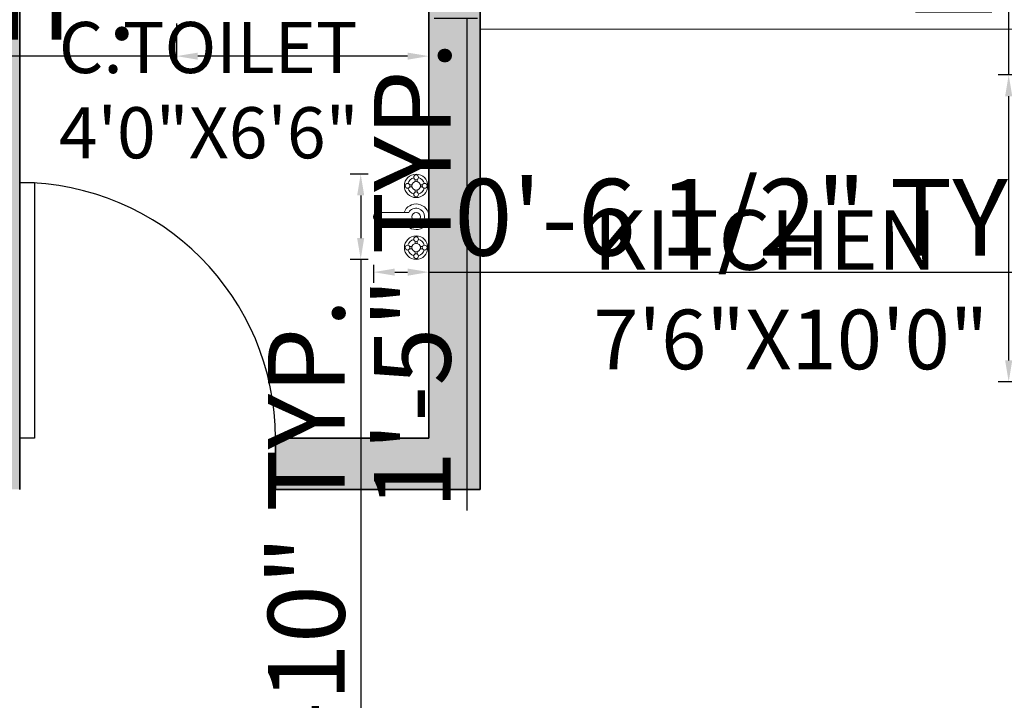
# Model space of a CAD drawing. Units: inches. Extents: x 2831 to 4250, y 1103 to 1797.
# Tile 6 of 15: x 3614 to 3730, y 1578 to 1658. Entities that reach past the tile are written whole.
import ezdxf

# ---------------------------------------------------------------- set-up
doc = ezdxf.new("R2010")
doc.units = ezdxf.units.IN
for name, color, linetype, lineweight in [('A-ANNO-DIMS', 2, 'Continuous', 18), ('A-AREA-IDEN', 7, 'Continuous', 18), ('A-DOOR', 4, 'Continuous', 25), ('A-FLOR-CASE', 9, 'Continuous', 18), ('A-WALL', 7, 'Continuous', 35), ('A-WALL-PATT', 252, 'Continuous', 13), ('Сантехника', 9, 'Continuous', 18)]:
    doc.layers.add(name, color=color, linetype=linetype, lineweight=lineweight)
doc.styles.get("Standard").update_dxf_attribs({"font": 'arial.ttf'})
doc.dimstyles.new('ISO-25', dxfattribs={"dimtxt": 9, "dimasz": 2.5, "dimexe": 1.25, "dimexo": 0.625, "dimtad": 1, "dimdec": 1, "dimlunit": 3, "dimtxsty": 'Standard', "dimcen": 2.5, "dimadec": 0, "dimazin": 0, "dimtfac": 1, "dimtdec": 1, "dimtmove": 0, "dimatfit": 3, "dimfxl": 1, "dimarcsym": 0})

# ---------------------------------------------------------------- blocks, each defined once
blk = doc.blocks.new('*U4')
for p, q in [((0, 0), (0, -6)), ((30, 0), (30, -6))]:
    blk.add_line(p, q)
blk.add_lwpolyline([(0, 0), (0, 30), (1.75, 30), (1.75, 0)], close=True)
blk.add_arc((0, 0), 30, 0, 90)
blk = doc.blocks.new('Faucet - Bathroom top')
for p, q in [((-4.107, 0.125), (-4.375, 0.125)), ((-3.75, 0.4788), (-3.75, 0.75)), ((-3.5, 0.482), (-3.5, 0.75)), ((-3.1461, 0.125), (-2.875, 0.125)), ((3.143, 0.125), (2.875, 0.125)), ((3.5, 0.4788), (3.5, 0.75)), ((3.75, 0.482), (3.75, 0.75)), ((4.1039, 0.125), (4.375, 0.125)), ((-4.1039, -0.125), (-4.375, -0.125)), ((-3.75, -0.4821), (-3.75, -0.75)), ((-3.5, -0.4789), (-3.5, -0.75)), ((-3.143, -0.125), (-2.875, -0.125)), ((-0.5, -0.8639), (-0.5, -4.5)), ((0.5, -4.5), (0.5, -0.8631)), ((3.1461, -0.125), (2.875, -0.125)), ((3.5, -0.4821), (3.5, -0.75)), ((3.75, -0.4789), (3.75, -0.75)), ((4.107, -0.125), (4.375, -0.125))]:
    blk.add_line(p, q)
for centre, radius in [((-3.625, 0), 1.375), ((-3.625, 1), 0.2795), ((3.625, 0), 1.375), ((3.625, 1), 0.2795), ((-4.625, 0), 0.2795), ((-3.625, 0), 0.5), ((-2.625, 0), 0.2795), ((0, 0), 0.5), ((2.625, 0), 0.2795), ((3.625, 0), 0.5), ((4.625, 0), 0.2795), ((-3.625, -1), 0.2795), ((3.625, -1), 0.2795)]:
    blk.add_circle(centre, radius)
for centre, radius, start, end in [((0, 0), 1.5, 289.6514, 250.3603), ((-3.625, 0), 1, 105.2407, 164.2093), ((-3.625, 0), 1, 16.44125, 74.07887), ((0, 0), 1, 300.3431, 239.7554), ((3.625, 0), 1, 106.12, 164.0884), ((3.625, 0), 1, 16.23422, 73.90469), ((-3.625, 0), 1, 196.2342, 253.9047), ((-3.625, 0), 1, 286.12, 344.0884), ((3.625, 0), 1, 196.4413, 254.0789), ((3.625, 0), 1, 285.2407, 344.2093), ((0, -4.5), 0.5, 180, 0)]:
    blk.add_arc(centre, radius, start, end)
blk = doc.blocks.new('*D77')
at = {"layer": 'A-ANNO-DIMS', "color": 0, "lineweight": -2, "transparency": 16777216}
for p, q in [((3512.23, 1679.89), (3512.23, 1668.46)), ((3584.23, 1679.89), (3584.23, 1668.46)), ((3514.73, 1669.71), (3581.73, 1669.71)), ((3584.23, 1669.71), (3701.86, 1669.71))]:
    blk.add_line(p, q, dxfattribs=at)
at = {"layer": 'A-ANNO-DIMS', "color": 0, "transparency": 16777216}
for points in [[(3514.73, 1670.13), (3514.73, 1669.3), (3512.23, 1669.71)], [(3581.73, 1670.13), (3581.73, 1669.3), (3584.23, 1669.71)]]:
    blk.add_solid(points, dxfattribs=at)
at = {"layer": 'Defpoints', "color": 0, "transparency": 16777216}
for p in [(3512.23, 1680.51), (3584.23, 1680.51), (3584.23, 1669.71)]:
    blk.add_point(p, dxfattribs=at)
at = {"layer": 'A-ANNO-DIMS', "color": 0, "transparency": 16777216, "insert": (3644.3, 1674.99), "char_height": 9, "attachment_point": 5}
blk.add_mtext('WINDOW 6\'-0" TYP.', dxfattribs=at)
blk = doc.blocks.new('*D85')
at = {"layer": 'A-ANNO-DIMS', "color": 0, "lineweight": -2, "transparency": 16777216}
for p, q in [((3730.24, 1651.15), (3730.24, 1797.34)), ((3735.01, 1651.15), (3728.99, 1651.15)), ((3730.24, 1617.65), (3730.24, 1648.65)), ((3735.01, 1615.15), (3728.99, 1615.15))]:
    blk.add_line(p, q, dxfattribs=at)
at = {"layer": 'A-ANNO-DIMS', "color": 0, "transparency": 16777216}
for points in [[(3729.82, 1648.65), (3730.66, 1648.65), (3730.24, 1651.15)], [(3729.82, 1617.65), (3730.66, 1617.65), (3730.24, 1615.15)]]:
    blk.add_solid(points, dxfattribs=at)
at = {"layer": 'Defpoints', "color": 0, "transparency": 16777216}
for p in [(3730.24, 1651.15), (3735.64, 1651.15), (3735.64, 1615.15)]:
    blk.add_point(p, dxfattribs=at)
at = {"layer": 'A-ANNO-DIMS', "color": 0, "transparency": 16777216, "insert": (3724.96, 1725.49), "char_height": 9, "attachment_point": 5, "rotation": 90}
blk.add_mtext('DOUBLE SINK 3\'-0" TYP.', dxfattribs=at)
blk = doc.blocks.new('*D87')
at = {"layer": 'A-ANNO-DIMS', "color": 0, "lineweight": -2, "transparency": 16777216}
for p, q in [((3649.73, 1552.52), (3649.73, 1560.11)), ((3696.18, 1552.52), (3696.18, 1560.11)), ((3652.23, 1558.86), (3693.68, 1558.86)), ((3696.18, 1558.86), (3813.01, 1558.86))]:
    blk.add_line(p, q, dxfattribs=at)
at = {"layer": 'A-ANNO-DIMS', "color": 0, "transparency": 16777216}
for points in [[(3652.23, 1559.28), (3652.23, 1558.44), (3649.73, 1558.86)], [(3693.68, 1559.28), (3693.68, 1558.44), (3696.18, 1558.86)]]:
    blk.add_solid(points, dxfattribs=at)
at = {"layer": 'Defpoints', "color": 0, "transparency": 16777216}
for p in [(3696.18, 1558.86), (3649.73, 1551.89), (3696.18, 1551.89)]:
    blk.add_point(p, dxfattribs=at)
at = {"layer": 'A-ANNO-DIMS', "color": 0, "transparency": 16777216, "insert": (3755.85, 1564.14), "char_height": 9, "attachment_point": 5}
blk.add_mtext('HOB 3\'-10 1/2" TYP.', dxfattribs=at)
blk = doc.blocks.new('*D89')
at = {"layer": 'A-ANNO-DIMS', "color": 0, "lineweight": -2, "transparency": 16777216}
for p, q in [((3632.62, 1657.17), (3632.62, 1652.11)), ((3662.23, 1657.17), (3662.23, 1652.11)), ((3632.62, 1653.36), (3528.23, 1653.36)), ((3659.73, 1653.36), (3635.12, 1653.36))]:
    blk.add_line(p, q, dxfattribs=at)
at = {"layer": 'A-ANNO-DIMS', "color": 0, "transparency": 16777216}
for points in [[(3635.12, 1653.77), (3635.12, 1652.94), (3632.62, 1653.36)], [(3659.73, 1653.77), (3659.73, 1652.94), (3662.23, 1653.36)]]:
    blk.add_solid(points, dxfattribs=at)
at = {"layer": 'Defpoints', "color": 0, "transparency": 16777216}
for p in [(3632.62, 1657.8), (3662.23, 1657.8), (3632.62, 1653.36)]:
    blk.add_point(p, dxfattribs=at)
at = {"layer": 'A-ANNO-DIMS', "color": 0, "transparency": 16777216, "insert": (3579.17, 1658.64), "char_height": 9, "attachment_point": 5}
blk.add_mtext('WC 2\'-5 1/2" TYP.', dxfattribs=at)
blk = doc.blocks.new('*D90')
at = {"layer": 'A-ANNO-DIMS', "color": 0, "lineweight": -2, "transparency": 16777216}
for p, q in [((3662.85, 1674.59), (3667.92, 1674.59)), ((3666.67, 1672.09), (3666.67, 1660.3)), ((3662.85, 1657.8), (3667.92, 1657.8)), ((3666.67, 1657.8), (3666.67, 1600.04))]:
    blk.add_line(p, q, dxfattribs=at)
at = {"layer": 'A-ANNO-DIMS', "color": 0, "transparency": 16777216}
for points in [[(3666.25, 1672.09), (3667.08, 1672.09), (3666.67, 1674.59)], [(3666.25, 1660.3), (3667.08, 1660.3), (3666.67, 1657.8)]]:
    blk.add_solid(points, dxfattribs=at)
at = {"layer": 'Defpoints', "color": 0, "transparency": 16777216}
for p in [(3662.23, 1674.59), (3662.23, 1657.8), (3666.67, 1657.8)]:
    blk.add_point(p, dxfattribs=at)
at = {"layer": 'A-ANNO-DIMS', "color": 0, "transparency": 16777216, "insert": (3661.45, 1627.67), "char_height": 9, "attachment_point": 5, "rotation": 90}
blk.add_mtext('1\'-5" TYP.', dxfattribs=at)
blk = doc.blocks.new('*D91')
at = {"layer": 'A-ANNO-DIMS', "color": 0, "lineweight": -2, "transparency": 16777216}
for p, q in [((3655.1, 1639.51), (3652.98, 1639.51)), ((3654.23, 1637.01), (3654.23, 1632.01)), ((3655.1, 1629.51), (3652.98, 1629.51)), ((3654.23, 1629.51), (3654.23, 1535.73))]:
    blk.add_line(p, q, dxfattribs=at)
at = {"layer": 'A-ANNO-DIMS', "color": 0, "transparency": 16777216}
for points in [[(3653.81, 1637.01), (3654.64, 1637.01), (3654.23, 1639.51)], [(3653.81, 1632.01), (3654.64, 1632.01), (3654.23, 1629.51)]]:
    blk.add_solid(points, dxfattribs=at)
at = {"layer": 'Defpoints', "color": 0, "transparency": 16777216}
for p in [(3655.73, 1639.51), (3654.23, 1629.51), (3655.73, 1629.51)]:
    blk.add_point(p, dxfattribs=at)
at = {"layer": 'A-ANNO-DIMS', "color": 0, "transparency": 16777216, "insert": (3649.01, 1581.37), "char_height": 9, "attachment_point": 5, "rotation": 90}
blk.add_mtext('TAP 0\'-10" TYP.', dxfattribs=at)
blk = doc.blocks.new('*D92')
at = {"layer": 'A-ANNO-DIMS', "color": 0, "lineweight": -2, "transparency": 16777216}
for p, q in [((3655.73, 1628.88), (3655.73, 1626.76)), ((3662.23, 1628.88), (3662.23, 1626.76)), ((3658.23, 1628.01), (3659.73, 1628.01)), ((3662.23, 1628.01), (3741.81, 1628.01))]:
    blk.add_line(p, q, dxfattribs=at)
at = {"layer": 'A-ANNO-DIMS', "color": 0, "transparency": 16777216}
for points in [[(3658.23, 1628.43), (3658.23, 1627.59), (3655.73, 1628.01)], [(3659.73, 1628.43), (3659.73, 1627.59), (3662.23, 1628.01)]]:
    blk.add_solid(points, dxfattribs=at)
at = {"layer": 'Defpoints', "color": 0, "transparency": 16777216}
for p in [(3655.73, 1629.51), (3662.23, 1629.51), (3662.23, 1628.01)]:
    blk.add_point(p, dxfattribs=at)
at = {"layer": 'A-ANNO-DIMS', "color": 0, "transparency": 16777216, "insert": (3703.27, 1633.29), "char_height": 9, "attachment_point": 5}
blk.add_mtext('0\'-6 1/2" TYP.', dxfattribs=at)

msp = doc.modelspace()

# ---------------------------------------------------------------- hatches: boundary and pattern name
at = {"layer": 'A-WALL-PATT'}
h = msp.add_hatch(color=256, dxfattribs=at)
h.dxf.hatch_style = 1
h.paths.add_polyline_path([(3479.23, 1418.51), (3488.23, 1418.51), (3488.23, 1426.81), (3488.23, 1460.51), (3588.23, 1460.51), (3588.23, 1466.51), (3488.23, 1466.51), (3488.23, 1470.51), (3479.23, 1470.51)])
h.paths.add_polyline_path([(3488.23, 1506.51), (3488.23, 1512.51), (3479.23, 1512.51), (3479.23, 1506.51)])
h.paths.add_polyline_path([(3488.23, 1370.51), (3479.23, 1370.51), (3479.23, 1319.51), (3521.23, 1319.51), (3521.23, 1328.51), (3488.23, 1328.51)])
h.paths.add_polyline_path([(3794.23, 1319.51), (3794.23, 1247.51), (3614.23, 1247.51), (3614.23, 1242.51), (3803.23, 1242.51), (3803.23, 1328.51), (3767.23, 1328.51), (3767.23, 1394.51), (3758.23, 1394.51), (3758.23, 1328.51), (3635.23, 1328.51), (3635.23, 1460.51), (3637.23, 1460.51), (3637.23, 1466.51), (3624.23, 1466.51), (3624.23, 1460.51), (3626.23, 1460.51), (3626.23, 1328.51), (3593.23, 1328.51), (3593.23, 1319.51)])
h.paths.add_polyline_path([(3758.23, 1460.51), (3758.23, 1442.51), (3767.23, 1442.51), (3767.23, 1460.51), (3783.23, 1460.51), (3783.23, 1492.51), (3774.23, 1492.51), (3774.23, 1466.51), (3761.32, 1466.51), (3726.23, 1466.51), (3726.23, 1468.51), (3720.23, 1468.51), (3720.23, 1466.51), (3673.23, 1466.51), (3673.23, 1460.51)])
h.paths.add_polyline_path([(3597.63, 1698.24), (3687.22, 1698.24), (3687.22, 1717.46), (3597.63, 1717.46)], flags=9)
h.paths.add_polyline_path([(3776.75, 1438.29), (3776.75, 1360.77), (3795.97, 1360.77), (3795.97, 1438.29)], flags=25)
h.paths.add_polyline_path([(3453.37, 1482.95), (3453.37, 1401.85), (3472.59, 1401.85), (3472.59, 1482.95)], flags=9)
h.paths.add_polyline_path([(3506.21, 1267.1), (3560.71, 1267.1), (3560.71, 1293.71), (3506.21, 1293.71)], flags=9)
h.paths.add_polyline_path([(3760.5, 1579.7), (3798.74, 1579.7), (3798.74, 1602.51), (3760.5, 1602.51)], flags=9)
h.paths.add_polyline_path([(3617, 1637.95), (3659.12, 1637.95), (3659.12, 1660.76), (3617, 1660.76)], flags=9)
h.paths.add_polyline_path([(3679.39, 1612.63), (3728.46, 1612.63), (3728.46, 1639.25), (3679.39, 1639.25)], flags=9)
h.paths.add_polyline_path([(3731.07, 1499.72), (3773.19, 1499.72), (3773.19, 1522.53), (3731.07, 1522.53)], flags=9)
h.paths.add_polyline_path([(3652.82, 1496.49), (3701.95, 1496.49), (3701.95, 1523.1), (3652.82, 1523.1)], flags=9)
h.paths.add_polyline_path([(3550.37, 1510.97), (3604.5, 1510.97), (3604.5, 1537.58), (3550.37, 1537.58)], flags=9)
h.paths.add_polyline_path([(3514.45, 1612.63), (3570.67, 1612.63), (3570.67, 1639.25), (3514.45, 1639.25)], flags=9)
h = msp.add_hatch(color=256, dxfattribs=at)
h.dxf.hatch_style = 1
h.paths.add_polyline_path([(3783.23, 1560.51), (3767.23, 1560.51), (3767.23, 1572.51), (3761.23, 1572.51), (3758.23, 1572.51), (3758.23, 1560.51), (3488.23, 1560.51), (3488.23, 1562.51), (3485.23, 1562.51), (3479.23, 1562.51), (3479.23, 1552.51), (3485.23, 1552.51), (3488.23, 1552.51), (3488.23, 1554.51), (3642.23, 1554.51), (3642.23, 1498.51), (3648.23, 1498.51), (3648.23, 1554.51), (3720.23, 1554.51), (3720.23, 1498.51), (3726.23, 1498.51), (3726.23, 1554.51), (3774.23, 1554.51), (3774.23, 1528.51), (3783.23, 1528.51)])
h.paths.add_polyline_path([(3767.23, 1689.51), (3728.23, 1689.51), (3728.23, 1680.51), (3758.23, 1680.51), (3758.23, 1602.51), (3767.23, 1602.51)])
h.paths.add_polyline_path([(3680.23, 1689.51), (3656.23, 1689.51), (3656.23, 1680.51), (3662.23, 1680.51), (3662.23, 1608.51), (3644.23, 1608.51), (3644.23, 1602.51), (3668.23, 1602.51), (3668.23, 1680.51), (3680.23, 1680.51)])
h.paths.add_polyline_path([(3620.23, 1689.51), (3584.23, 1689.51), (3584.23, 1680.51), (3608.23, 1680.51), (3608.23, 1602.51), (3614.23, 1602.51), (3614.23, 1608.51), (3614.23, 1638.51), (3614.23, 1680.51), (3620.23, 1680.51)])
h.paths.add_polyline_path([(3512.23, 1689.51), (3479.23, 1689.51), (3479.23, 1665.51), (3488.23, 1665.51), (3488.23, 1680.51), (3512.23, 1680.51)])
h.paths.add_polyline_path([(3488.23, 1617.51), (3479.23, 1617.51), (3479.23, 1602.51), (3485.23, 1602.51), (3488.23, 1602.51)])

# ---------------------------------------------------------------- linework, layer by layer
at = {"layer": 'A-FLOR-CASE'}
msp.add_line((3668.23, 1656.51), (3734.23, 1656.51), dxfattribs=at)
at = {"layer": 'A-WALL'}
for p, q in [((3614.23, 1602.51), (3614.23, 1680.51)), ((3662.23, 1608.51), (3662.23, 1680.51)), ((3668.23, 1602.51), (3668.23, 1680.51)), ((3644.23, 1608.51), (3662.23, 1608.51)), ((3644.23, 1602.51), (3644.23, 1608.51)), ((3644.23, 1602.51), (3668.23, 1602.51))]:
    msp.add_line(p, q, dxfattribs=at)

# ---------------------------------------------------------------- block references
at = {"layer": 'A-DOOR'}
msp.add_blockref('*U4', (3614.23, 1608.51), dxfattribs=at)
at = {"layer": 'Сантехника', "rotation": 270}
msp.add_blockref('Faucet - Bathroom top', (3660.73, 1634.51), dxfattribs=at)

# ---------------------------------------------------------------- texts
at = {"layer": 'A-AREA-IDEN', "attachment_point": 1}
for s, insert, char_height in [('{\\fTimes New Roman|b0|i0|c0|p18;C.TOILET\\P4\'0"X6\'6"}', (3618.82, 1657.37), 6), ('{\\fTimes New Roman|b0|i0|c0|p18;KITCHEN\\P7\'6"X10\'0"}', (3681.52, 1635.28), 7)]:
    msp.add_mtext_dynamic_manual_height_columns(s, width=81.5075, gutter_width=12.5, heights=[0], dxfattribs=dict(at, insert=insert, char_height=char_height))

# ---------------------------------------------------------------- dimensions: what is measured, and where the dimension line sits
at = {"layer": 'A-ANNO-DIMS'}
for base, p1, p2, angle, text, picture, middle in [((3730.24, 1651.15), (3735.64, 1615.15), (3735.64, 1651.15), 90, 'DOUBLE SINK <> TYP.', '*D85', (3724.96, 1725.49)), ((3632.62, 1653.36), (3662.23, 1657.8), (3632.62, 1657.8), 180, 'WC <> TYP.', '*D89', (3579.17, 1658.64)), ((3666.67, 1657.8), (3662.23, 1674.59), (3662.23, 1657.8), 270, '<> TYP.', '*D90', (3661.45, 1627.67)), ((3654.23, 1629.51), (3655.73, 1639.51), (3655.73, 1629.51), 270, 'TAP <> TYP.', '*D91', (3649.01, 1581.37))]:
    dim = msp.add_linear_dim(base=base, p1=p1, p2=p2, angle=angle, text=text, dimstyle='ISO-25', override={"dimdec": 1, "dimlfac": 1, "dimrnd": 0, "dimzin": 1, "dimdsep": 46, "dimlunit": 4, "dimfrac": 2}, dxfattribs=at)
    dim.commit()
    dim.dimension.update_dxf_attribs({"geometry": picture, "text_midpoint": middle})
for base, p1, p2, text, picture, middle in [((3584.23, 1669.71), (3512.23, 1680.51), (3584.23, 1680.51), 'WINDOW <> TYP.', '*D77', (3644.3, 1674.99)), ((3662.23, 1628.01), (3655.73, 1629.51), (3662.23, 1629.51), '<> TYP.', '*D92', (3703.27, 1633.29)), ((3696.1815, 1558.8587), (3649.7349, 1551.8917), (3696.1815, 1551.8917), 'HOB <> TYP.', '*D87', (3755.845, 1564.1433))]:
    dim = msp.add_linear_dim(base=base, p1=p1, p2=p2, text=text, dimstyle='ISO-25', override={"dimdec": 1, "dimlfac": 1, "dimrnd": 0, "dimzin": 1, "dimdsep": 46, "dimlunit": 4, "dimfrac": 2}, dxfattribs=at)
    dim.commit()
    dim.dimension.update_dxf_attribs({"geometry": picture, "text_midpoint": middle})

doc.saveas('drawing.dxf')
